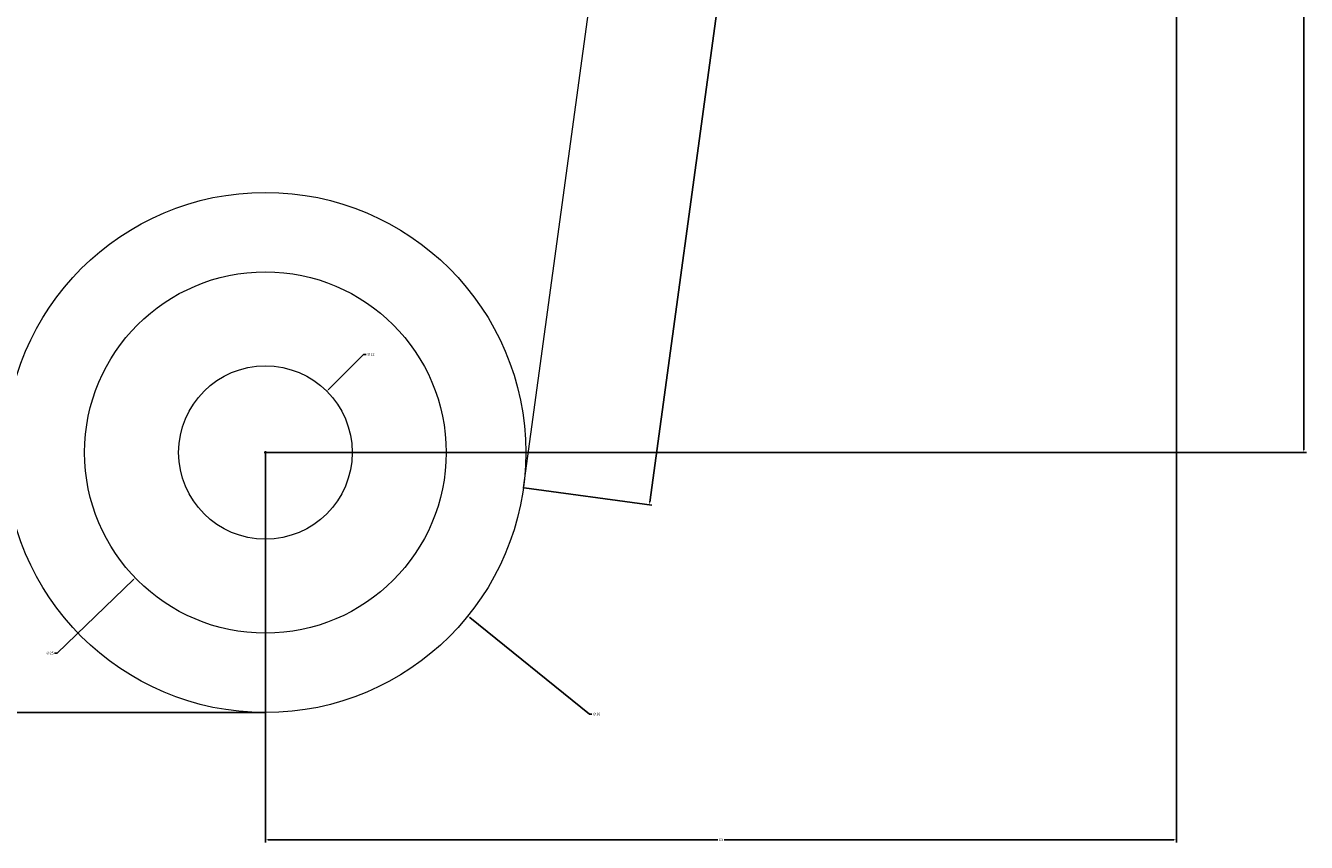
# Model space of a CAD drawing. Units: millimetres. Extents: x -9 to 135, y -119 to 27.
# Tile 2 of 12: x 46 to 135, y -119 to -63. Entities that reach past the tile are written whole.
import ezdxf

# ---------------------------------------------------------------- set-up
doc = ezdxf.new("R2010")
doc.units = ezdxf.units.MM
doc.layers.add('M-CONS', color=8, linetype='Continuous', lineweight=18)
doc.layers.add('M-DIMS', color=2, linetype='Continuous', lineweight=18)
doc.styles.get("Standard").update_dxf_attribs({"font": 'arial.ttf'})
doc.dimstyles.get("Standard").update_dxf_attribs({"dimtxt": 0.18, "dimasz": 0.18, "dimexe": 0.18, "dimexo": 0.0625, "dimgap": 0.09, "dimtad": 0, "dimtih": 1, "dimtoh": 1, "dimdec": 4, "dimzin": 0, "dimdsep": 46, "dimtxsty": 'Standard', "dimcen": 0.09, "dimadec": 0, "dimazin": 0, "dimtfac": 1, "dimtdec": 4, "dimtofl": 0, "dimtmove": 0, "dimatfit": 3, "dimfxl": 1, "dimtolj": 1, "dimtzin": 0, "dimarcsym": 0})

# ---------------------------------------------------------------- blocks, each defined once
blk = doc.blocks.new('*D3')
at = {"layer": 'Defpoints', "color": 0, "transparency": 16777216}
for p in [(0, 17.733), (-8.8, -110.267), (63, -110.267)]:
    blk.add_point(p, dxfattribs=at)
at = {"layer": 'M-DIMS', "color": 0, "lineweight": -2, "transparency": 16777216}
for p, q in [((-0.062, 17.733), (-8.98, 17.733)), ((-8.8, 17.553), (-8.8, -46.085)), ((-8.8, -110.087), (-8.8, -46.449)), ((62.938, -110.267), (-8.98, -110.267))]:
    blk.add_line(p, q, dxfattribs=at)
at = {"layer": 'M-DIMS', "color": 0, "transparency": 16777216}
for points in [[(-8.83, 17.553), (-8.77, 17.553), (-8.8, 17.733)], [(-8.83, -110.087), (-8.77, -110.087), (-8.8, -110.267)]]:
    blk.add_solid(points, dxfattribs=at)
at = {"layer": 'M-DIMS', "color": 0, "transparency": 16777216, "insert": (-8.8, -46.267), "char_height": 0.18, "attachment_point": 5}
blk.add_mtext('\\A1;128', dxfattribs=at)
blk = doc.blocks.new('*D13')
at = {"layer": 'Defpoints', "color": 0, "transparency": 16777216}
for p in [(126, 1.733), (63, -92.267), (134.8, -92.267)]:
    blk.add_point(p, dxfattribs=at)
at = {"layer": 'M-DIMS', "color": 0, "lineweight": -2, "transparency": 16777216}
for p, q in [((126.062, 1.733), (134.98, 1.733)), ((134.8, 1.553), (134.8, -45.085)), ((134.8, -92.087), (134.8, -45.449)), ((63.063, -92.267), (134.98, -92.267))]:
    blk.add_line(p, q, dxfattribs=at)
at = {"layer": 'M-DIMS', "color": 0, "transparency": 16777216}
for points in [[(134.77, 1.553), (134.83, 1.553), (134.8, 1.733)], [(134.77, -92.087), (134.83, -92.087), (134.8, -92.267)]]:
    blk.add_solid(points, dxfattribs=at)
at = {"layer": 'M-DIMS', "color": 0, "transparency": 16777216, "insert": (134.8, -45.267), "char_height": 0.18, "attachment_point": 5}
blk.add_mtext('\\A1;94', dxfattribs=at)
blk = doc.blocks.new('*D15')
at = {"layer": 'Defpoints', "color": 0, "transparency": 16777216}
for p in [(94, 1.733), (80.835, -94.702), (89.554, -95.892)]:
    blk.add_point(p, dxfattribs=at)
at = {"layer": 'M-DIMS', "color": 0, "lineweight": -2, "transparency": 16777216}
for p, q in [((94.062, 1.725), (102.897, 0.519)), ((102.695, 0.365), (96.161, -47.493)), ((89.578, -95.714), (96.112, -47.856)), ((80.896, -94.71), (89.732, -95.916))]:
    blk.add_line(p, q, dxfattribs=at)
at = {"layer": 'M-DIMS', "color": 0, "transparency": 16777216}
for points in [[(102.665, 0.369), (102.724, 0.36), (102.719, 0.543)], [(89.548, -95.71), (89.608, -95.718), (89.554, -95.892)]]:
    blk.add_solid(points, dxfattribs=at)
at = {"layer": 'M-DIMS', "color": 0, "transparency": 16777216, "insert": (96.136, -47.675), "char_height": 0.18, "attachment_point": 5}
blk.add_mtext('\\A1;97.33', dxfattribs=at)
blk = doc.blocks.new('*D16')
at = {"layer": 'Defpoints', "color": 0, "transparency": 16777216}
for p in [(126, 1.733), (63, -92.267), (126, -119.067)]:
    blk.add_point(p, dxfattribs=at)
at = {"layer": 'M-DIMS', "color": 0, "lineweight": -2, "transparency": 16777216}
for p, q in [((126, 1.671), (126, -119.247)), ((63, -92.329), (63, -119.247)), ((63.18, -119.067), (94.281, -119.067)), ((125.82, -119.067), (94.719, -119.067))]:
    blk.add_line(p, q, dxfattribs=at)
at = {"layer": 'M-DIMS', "color": 0, "transparency": 16777216}
for points in [[(63.18, -119.037), (63.18, -119.097), (63, -119.067)], [(125.82, -119.037), (125.82, -119.097), (126, -119.067)]]:
    blk.add_solid(points, dxfattribs=at)
at = {"layer": 'M-DIMS', "color": 0, "transparency": 16777216, "insert": (94.5, -119.067), "char_height": 0.18, "attachment_point": 5}
blk.add_mtext('\\A1;63', dxfattribs=at)
blk = doc.blocks.new('*D17')
at = {"layer": 'Defpoints', "color": 0, "transparency": 16777216}
for p in [(49, -80.953), (77, -103.58)]:
    blk.add_point(p, dxfattribs=at)
at = {"layer": 'M-DIMS', "color": 0, "lineweight": -2, "transparency": 16777216}
for p, q in [((62.91, -92.267), (63.09, -92.267)), ((63, -92.357), (63, -92.177)), ((85.4, -110.368), (77.14, -103.693)), ((85.58, -110.368), (85.4, -110.368))]:
    blk.add_line(p, q, dxfattribs=at)
at = {"layer": 'M-DIMS', "color": 0, "transparency": 16777216}
blk.add_solid([(77.159, -103.67), (77.121, -103.717), (77, -103.58)], dxfattribs=at)
at = {"layer": 'M-DIMS', "color": 0, "transparency": 16777216, "insert": (85.897, -110.368), "char_height": 0.18, "attachment_point": 5}
blk.add_mtext('\\A1;∅36', dxfattribs=at)
blk = doc.blocks.new('*D18')
at = {"layer": 'Defpoints', "color": 0, "transparency": 16777216}
for p in [(72.001, -83.593), (53.999, -100.941)]:
    blk.add_point(p, dxfattribs=at)
at = {"layer": 'M-DIMS', "color": 0, "lineweight": -2, "transparency": 16777216}
for p, q in [((62.91, -92.267), (63.09, -92.267)), ((63, -92.357), (63, -92.177)), ((48.599, -106.145), (53.87, -101.066)), ((48.419, -106.145), (48.599, -106.145))]:
    blk.add_line(p, q, dxfattribs=at)
at = {"layer": 'M-DIMS', "color": 0, "transparency": 16777216}
blk.add_solid([(53.849, -101.044), (53.89, -101.087), (53.999, -100.941)], dxfattribs=at)
at = {"layer": 'M-DIMS', "color": 0, "transparency": 16777216, "insert": (48.101, -106.145), "char_height": 0.18, "attachment_point": 5}
blk.add_mtext('\\A1;∅25', dxfattribs=at)
blk = doc.blocks.new('*D19')
at = {"layer": 'Defpoints', "color": 0, "transparency": 16777216}
for p in [(67.243, -88.024), (58.757, -96.509)]:
    blk.add_point(p, dxfattribs=at)
at = {"layer": 'M-DIMS', "color": 0, "lineweight": -2, "transparency": 16777216}
for p, q in [((69.788, -85.479), (67.37, -87.897)), ((69.968, -85.479), (69.788, -85.479)), ((62.91, -92.267), (63.09, -92.267)), ((63, -92.357), (63, -92.177))]:
    blk.add_line(p, q, dxfattribs=at)
at = {"layer": 'M-DIMS', "color": 0, "transparency": 16777216}
blk.add_solid([(67.349, -87.876), (67.391, -87.918), (67.243, -88.024)], dxfattribs=at)
at = {"layer": 'M-DIMS', "color": 0, "transparency": 16777216, "insert": (70.284, -85.479), "char_height": 0.18, "attachment_point": 5}
blk.add_mtext('\\A1;∅12', dxfattribs=at)

msp = doc.modelspace()

# ---------------------------------------------------------------- linework, layer by layer
at = {"layer": 'M-CONS'}
msp.add_line((94, 1.733, 115.129), (80.835, -94.702, 115.129), dxfattribs=at)
for radius in [18, 12.5, 6]:
    msp.add_circle((63, -92.267, 115.129), radius, dxfattribs=at)

# ---------------------------------------------------------------- dimensions: what is measured, and where the dimension line sits
at = {"layer": 'M-DIMS'}
for base, p1, p2, angle, override, picture, middle in [((-8.8, -110.267), (0, 17.733), (63, -110.267), 90, {"dimdec": 0, "dimlfac": 1, "dimrnd": 0, "dimzin": 0, "dimdsep": 46, "dimlunit": 2}, '*D3', (-8.8, -46.267)), ((134.8, -92.267), (126, 1.733), (63, -92.267), 90, {"dimdec": 0, "dimlfac": 1, "dimrnd": 0, "dimzin": 0, "dimdsep": 46, "dimlunit": 2}, '*D13', (134.8, -45.267)), ((89.554, -95.892), (94, 1.733), (80.835, -94.702), 262.22595, {"dimdec": 2, "dimlfac": 1, "dimrnd": 0, "dimzin": 0, "dimdsep": 46, "dimlunit": 2}, '*D15', (96.136, -47.675))]:
    dim = msp.add_linear_dim(base=base, p1=p1, p2=p2, angle=angle, dimstyle='Standard', override=override, dxfattribs=at)
    dim.commit()
    dim.dimension.update_dxf_attribs({"geometry": picture, "text_midpoint": middle})
dim = msp.add_linear_dim(base=(126, -119.067), p1=(63, -92.267), p2=(126, 1.733), dimstyle='Standard', override={"dimdec": 0, "dimlfac": 1, "dimrnd": 0, "dimzin": 0, "dimdsep": 46, "dimlunit": 2}, dxfattribs=at)
dim.commit()
dim.dimension.update_dxf_attribs({"geometry": '*D16', "text_midpoint": (94.5, -119.067)})
for p1, p2, picture, middle in [((49, -80.953), (77, -103.58), '*D17', (85.897, -110.368)), ((72.001, -83.593), (53.999, -100.941), '*D18', (48.101, -106.145)), ((58.757, -96.509), (67.243, -88.024), '*D19', (70.284, -85.479))]:
    dim = msp.add_diameter_dim_2p(p1=p1, p2=p2, dimstyle='Standard', override={"dimdec": 0, "dimlfac": 1, "dimrnd": 0, "dimzin": 0, "dimdsep": 46, "dimlunit": 2}, dxfattribs=at)
    dim.commit()
    dim.dimension.update_dxf_attribs({"geometry": picture, "text_midpoint": middle, "dimtype": 163})

doc.saveas('drawing.dxf')
